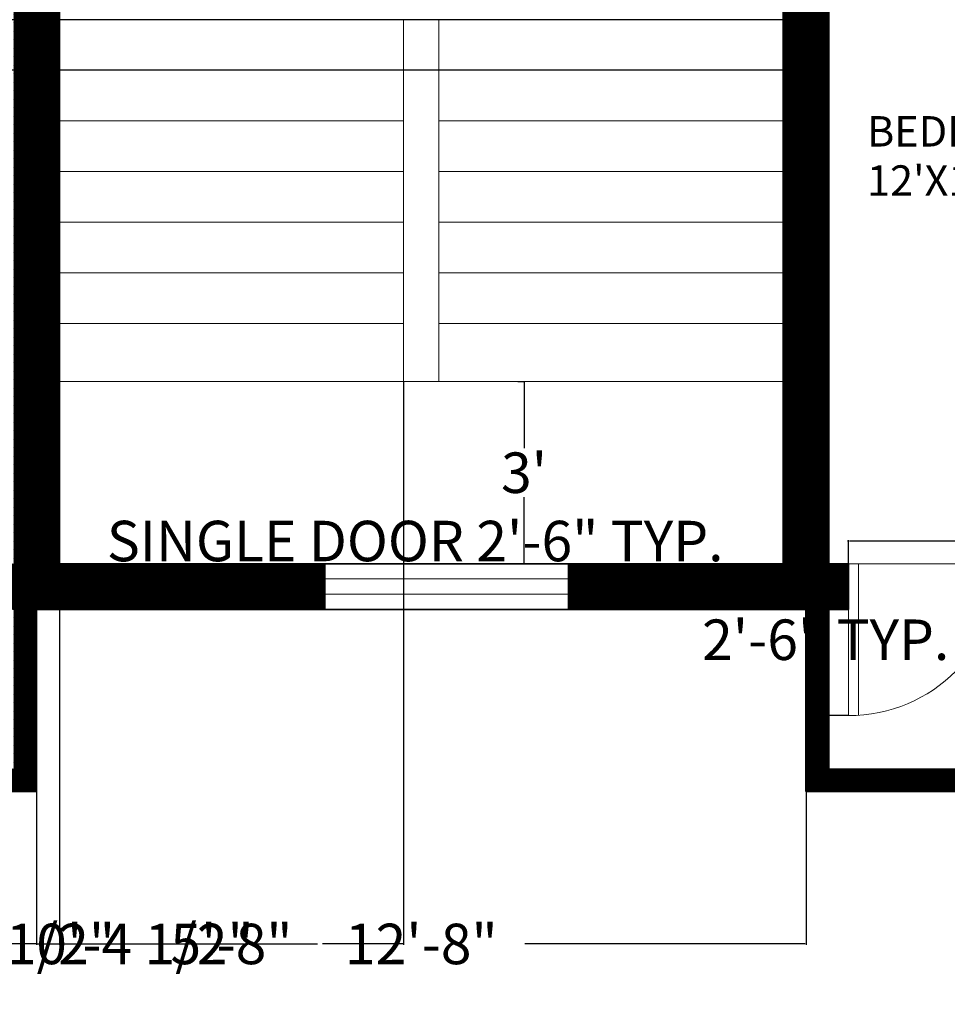
# Model space of a CAD drawing. Units: inches. Extents: x 108 to 771, y 58 to 590.
# Tile 3 of 8: x 341 to 524, y 58 to 253. Entities that reach past the tile are written whole.
import ezdxf

# ---------------------------------------------------------------- set-up
doc = ezdxf.new("R2010")
doc.units = ezdxf.units.IN
doc.header["$MEASUREMENT"] = 0
for name, color, linetype, lineweight in [('A-ANNO-DIMS', 2, 'Continuous', 13), ('A-AREA-IDEN', 7, 'Continuous', 18), ('A-DOOR', 3, 'Continuous', 18), ('A-FLOR-STRS', 7, 'Continuous', 18), ('A-GLAZ', 4, 'Continuous', 18), ('A-WALL', 7, 'Continuous', 35), ('A-WALL-PATT', 252, 'Continuous', 9)]:
    doc.layers.add(name, color=color, linetype=linetype, lineweight=lineweight)
doc.styles.get("Standard").update_dxf_attribs({"font": 'italic8.shx'})
doc.dimstyles.get("Standard").update_dxf_attribs({"dimtxt": 8, "dimasz": 0.18, "dimexe": 0.18, "dimexo": 0.0625, "dimgap": 0.09, "dimtad": 0, "dimtih": 1, "dimtoh": 1, "dimzin": 0, "dimdsep": 46, "dimlunit": 3, "dimtxsty": 'Standard', "dimcen": 0.09, "dimclrt": 6, "dimadec": 0, "dimazin": 0, "dimtfac": 1, "dimtofl": 0, "dimtmove": 0, "dimatfit": 3, "dimfxl": 1, "dimtolj": 1, "dimtzin": 0, "dimarcsym": 0})

# ---------------------------------------------------------------- blocks, each defined once
blk = doc.blocks.new('*D4')
at = {"layer": 'A-ANNO-DIMS', "color": 0, "lineweight": -2, "transparency": 16777216}
for p, q in [((438.9, 181.05), (440.33, 181.05)), ((440.15, 180.87), (440.15, 167.9)), ((440.15, 145.23), (440.15, 158.2)), ((438.9, 145.05), (440.33, 145.05))]:
    blk.add_line(p, q, dxfattribs=at)
at = {"layer": 'A-ANNO-DIMS', "color": 0, "transparency": 16777216}
for points in [[(440.12, 180.87), (440.18, 180.87), (440.15, 181.05)], [(440.12, 145.23), (440.18, 145.23), (440.15, 145.05)]]:
    blk.add_solid(points, dxfattribs=at)
at = {"layer": 'Defpoints', "color": 0, "transparency": 16777216}
for p in [(438.84, 181.05), (438.84, 145.05), (440.15, 145.05)]:
    blk.add_point(p, dxfattribs=at)
at = {"layer": 'A-ANNO-DIMS', "color": 0, "transparency": 16777216, "insert": (440.15, 163.05), "char_height": 8, "attachment_point": 5}
blk.add_mtext("\\A1;3'", dxfattribs=at)
blk = doc.blocks.new('DOOR-SINGLE-30')
for p, q in [((28, 29.93), (28, 0)), ((30, 30), (30, 0)), ((30, 0), (0, 0))]:
    blk.add_line(p, q)
blk.add_arc((30, 0), 30, 90, 180)
blk = doc.blocks.new('WINDOW-48')
for p, q in [((0, 48), (0, 0)), ((9, 48), (0, 48)), ((3, 48), (3, 0)), ((6, 48), (6, 0)), ((9, 0), (9, 48)), ((0, 0), (9, 0))]:
    blk.add_line(p, q)
blk = doc.blocks.new('*D24')
at = {"layer": 'A-ANNO-DIMS', "color": 0, "lineweight": -2, "transparency": 16777216}
for p, q in [((504.24, 149.55), (504.06, 149.55)), ((504.24, 145.12), (504.24, 149.73)), ((534.06, 149.55), (504.42, 149.55)), ((534.24, 145.12), (534.24, 149.73))]:
    blk.add_line(p, q, dxfattribs=at)
at = {"layer": 'A-ANNO-DIMS', "color": 0, "transparency": 16777216}
for points in [[(504.42, 149.58), (504.42, 149.52), (504.24, 149.55)], [(534.06, 149.58), (534.06, 149.52), (534.24, 149.55)]]:
    blk.add_solid(points, dxfattribs=at)
at = {"layer": 'Defpoints', "color": 0, "transparency": 16777216}
for p in [(504.24, 149.55), (504.24, 145.05), (534.24, 145.05)]:
    blk.add_point(p, dxfattribs=at)
at = {"layer": 'A-ANNO-DIMS', "color": 6, "transparency": 16777216, "insert": (418.64, 149.55), "char_height": 8, "attachment_point": 5}
blk.add_mtext('\\A1;SINGLE DOOR 2\'-6" TYP.', dxfattribs=at)
blk = doc.blocks.new('*D25')
at = {"layer": 'A-ANNO-DIMS', "color": 0, "lineweight": -2, "transparency": 16777216}
for p, q in [((504.18, 145.05), (499.56, 145.05)), ((499.74, 144.87), (499.74, 134.9)), ((499.74, 115.23), (499.74, 125.2)), ((504.18, 115.05), (499.56, 115.05))]:
    blk.add_line(p, q, dxfattribs=at)
at = {"layer": 'A-ANNO-DIMS', "color": 0, "transparency": 16777216}
for points in [[(499.71, 144.87), (499.77, 144.87), (499.74, 145.05)], [(499.71, 115.23), (499.77, 115.23), (499.74, 115.05)]]:
    blk.add_solid(points, dxfattribs=at)
at = {"layer": 'Defpoints', "color": 0, "transparency": 16777216}
for p in [(504.24, 145.05), (499.74, 115.05), (504.24, 115.05)]:
    blk.add_point(p, dxfattribs=at)
at = {"layer": 'A-ANNO-DIMS', "color": 6, "transparency": 16777216, "insert": (499.74, 130.05), "char_height": 8, "attachment_point": 5}
blk.add_mtext('\\A1;2\'-6" TYP.', dxfattribs=at)
blk = doc.blocks.new('*D46')
at = {"layer": 'A-ANNO-DIMS', "color": 0, "lineweight": -2, "transparency": 16777216}
for p, q in [((162.35, 99.99), (162.35, 69.77)), ((343.85, 99.99), (343.85, 69.77)), ((162.53, 69.95), (218.72, 69.95)), ((343.67, 69.95), (287.47, 69.95))]:
    blk.add_line(p, q, dxfattribs=at)
at = {"layer": 'A-ANNO-DIMS', "color": 0, "transparency": 16777216}
for points in [[(162.53, 69.98), (162.53, 69.92), (162.35, 69.95)], [(343.67, 69.98), (343.67, 69.92), (343.85, 69.95)]]:
    blk.add_solid(points, dxfattribs=at)
at = {"layer": 'Defpoints', "color": 0, "transparency": 16777216}
for p in [(162.35, 100.05), (343.85, 100.05), (343.85, 69.95)]:
    blk.add_point(p, dxfattribs=at)
at = {"layer": 'A-ANNO-DIMS', "color": 6, "transparency": 16777216, "insert": (253.1, 69.95), "char_height": 8, "attachment_point": 5}
blk.add_mtext('\\A1;15\'-1 1/2"', dxfattribs=at)
blk = doc.blocks.new('*D47')
at = {"layer": 'A-ANNO-DIMS', "color": 0, "lineweight": -2, "transparency": 16777216}
for p, q in [((343.85, 99.99), (343.85, 69.77)), ((495.85, 99.99), (495.85, 69.77)), ((344.03, 69.95), (399.37, 69.95)), ((495.67, 69.95), (440.32, 69.95))]:
    blk.add_line(p, q, dxfattribs=at)
at = {"layer": 'A-ANNO-DIMS', "color": 0, "transparency": 16777216}
for points in [[(344.03, 69.98), (344.03, 69.92), (343.85, 69.95)], [(495.67, 69.98), (495.67, 69.92), (495.85, 69.95)]]:
    blk.add_solid(points, dxfattribs=at)
at = {"layer": 'Defpoints', "color": 0, "transparency": 16777216}
for p in [(343.85, 100.05), (495.85, 100.05), (495.85, 69.95)]:
    blk.add_point(p, dxfattribs=at)
at = {"layer": 'A-ANNO-DIMS', "color": 6, "transparency": 16777216, "insert": (419.85, 69.95), "char_height": 8, "attachment_point": 5}
blk.add_mtext('\\A1;12\'-8"', dxfattribs=at)
blk = doc.blocks.new('*D52')
at = {"layer": 'A-ANNO-DIMS', "color": 0, "lineweight": -2, "transparency": 16777216}
for p, q in [((348.35, 145.12), (348.35, 578.33)), ((348.53, 578.15), (399.37, 578.15)), ((491.17, 578.15), (440.32, 578.15)), ((491.35, 145.12), (491.35, 578.33))]:
    blk.add_line(p, q, dxfattribs=at)
at = {"layer": 'A-ANNO-DIMS', "color": 0, "transparency": 16777216}
for points in [[(348.53, 578.18), (348.53, 578.12), (348.35, 578.15)], [(491.17, 578.18), (491.17, 578.12), (491.35, 578.15)]]:
    blk.add_solid(points, dxfattribs=at)
at = {"layer": 'Defpoints', "color": 0, "transparency": 16777216}
for p in [(491.35, 578.15), (348.35, 145.05), (491.35, 145.05)]:
    blk.add_point(p, dxfattribs=at)
at = {"layer": 'A-ANNO-DIMS', "color": 6, "transparency": 16777216, "insert": (419.85, 578.15), "char_height": 8, "attachment_point": 5}
blk.add_mtext('\\A1;11\'-11"', dxfattribs=at)
blk = doc.blocks.new('*D59')
at = {"layer": 'A-ANNO-DIMS', "color": 0, "lineweight": -2, "transparency": 16777216}
for p, q in [((327.35, 538.99), (327.35, 69.77)), ((331.85, 538.99), (331.85, 69.77)), ((327.53, 69.95), (331.67, 69.95)), ((331.85, 69.95), (332.03, 69.95))]:
    blk.add_line(p, q, dxfattribs=at)
at = {"layer": 'A-ANNO-DIMS', "color": 0, "transparency": 16777216}
for points in [[(327.53, 69.98), (327.53, 69.92), (327.35, 69.95)], [(331.67, 69.98), (331.67, 69.92), (331.85, 69.95)]]:
    blk.add_solid(points, dxfattribs=at)
at = {"layer": 'Defpoints', "color": 0, "transparency": 16777216}
for p in [(327.35, 539.05), (331.85, 539.05), (331.85, 69.95)]:
    blk.add_point(p, dxfattribs=at)
at = {"layer": 'A-ANNO-DIMS', "color": 6, "transparency": 16777216, "insert": (365.26, 69.95), "char_height": 8, "attachment_point": 5}
blk.add_mtext('\\A1;0\'-4 1/2"', dxfattribs=at)
blk = doc.blocks.new('*D61')
at = {"layer": 'A-ANNO-DIMS', "color": 0, "lineweight": -2, "transparency": 16777216}
for p, q in [((132.245389, 252.733083), (132.245389, 252.913083)), ((491.282889, 252.553083), (132.065389, 252.553083)), ((491.282889, 242.553083), (132.065389, 242.553083)), ((132.245389, 242.373083), (132.245389, 242.193083))]:
    blk.add_line(p, q, dxfattribs=at)
at = {"layer": 'A-ANNO-DIMS', "color": 0, "transparency": 16777216}
for points in [[(132.215389, 252.733083), (132.275389, 252.733083), (132.245389, 252.553083)], [(132.215389, 242.373083), (132.275389, 242.373083), (132.245389, 242.553083)]]:
    blk.add_solid(points, dxfattribs=at)
at = {"layer": 'Defpoints', "color": 0, "transparency": 16777216}
for p in [(491.345389, 252.553083), (132.245389, 242.553083), (491.345389, 242.553083)]:
    blk.add_point(p, dxfattribs=at)
at = {"layer": 'A-ANNO-DIMS', "color": 6, "transparency": 16777216, "insert": (132.245389, 247.553083), "char_height": 8, "attachment_point": 5}
blk.add_mtext('\\A1;0\'-10"', dxfattribs=at)
blk = doc.blocks.new('*D66')
at = {"layer": 'A-ANNO-DIMS', "color": 0, "lineweight": -2, "transparency": 16777216}
for p, q in [((348.35, 180.99), (348.35, 69.77)), ((416.35, 180.99), (416.35, 69.77)), ((348.53, 69.95), (364.35, 69.95)), ((416.17, 69.95), (400.34, 69.95))]:
    blk.add_line(p, q, dxfattribs=at)
at = {"layer": 'A-ANNO-DIMS', "color": 0, "transparency": 16777216}
for points in [[(348.53, 69.98), (348.53, 69.92), (348.35, 69.95)], [(416.17, 69.98), (416.17, 69.92), (416.35, 69.95)]]:
    blk.add_solid(points, dxfattribs=at)
at = {"layer": 'Defpoints', "color": 0, "transparency": 16777216}
for p in [(348.35, 181.05), (416.35, 181.05), (416.35, 69.95)]:
    blk.add_point(p, dxfattribs=at)
at = {"layer": 'A-ANNO-DIMS', "color": 6, "transparency": 16777216, "insert": (382.35, 69.95), "char_height": 8, "attachment_point": 5}
blk.add_mtext('\\A1;5\'-8"', dxfattribs=at)
blk = doc.blocks.new('*D68')
at = {"layer": 'A-ANNO-DIMS', "color": 0, "lineweight": -2, "transparency": 16777216}
for p, q in [((259.84, 135.99), (259.84, 69.77)), ((304.47, 135.99), (304.47, 69.77)), ((260.02, 69.95), (304.29, 69.95)), ((304.47, 69.95), (304.65, 69.95))]:
    blk.add_line(p, q, dxfattribs=at)
at = {"layer": 'A-ANNO-DIMS', "color": 0, "transparency": 16777216}
for points in [[(260.02, 69.98), (260.02, 69.92), (259.84, 69.95)], [(304.29, 69.98), (304.29, 69.92), (304.47, 69.95)]]:
    blk.add_solid(points, dxfattribs=at)
at = {"layer": 'Defpoints', "color": 0, "transparency": 16777216}
for p in [(259.84, 136.05), (304.47, 136.05), (304.47, 69.95)]:
    blk.add_point(p, dxfattribs=at)
at = {"layer": 'A-ANNO-DIMS', "color": 6, "transparency": 16777216, "insert": (337.88, 69.95), "char_height": 8, "attachment_point": 5}
blk.add_mtext('\\A1;3\'-8 1/2"', dxfattribs=at)

msp = doc.modelspace()

# ---------------------------------------------------------------- hatches: boundary and pattern name
at = {"layer": 'A-WALL-PATT'}
h = msp.add_hatch(dxfattribs=at)
h.set_pattern_fill('ANSI31', color=256)
h.paths.add_polyline_path([(171.345, 461.548), (162.345, 461.548), (162.345, 390.901), (171.345, 390.901), (171.345, 393.51), (171.345, 402.553), (233.142, 402.553), (233.142, 407.053), (171.345, 407.053)])
h.paths.add_polyline_path([(331.845, 438.553), (336.68, 438.554), (336.68, 443.053), (331.845, 443.053), (331.845, 539.053), (365.02, 539.053), (365.02, 548.053), (280.772, 548.053), (280.772, 539.053), (327.345, 539.053), (327.345, 407.053), (325.63, 407.053), (325.63, 402.553), (331.845, 402.553)])
h.paths.add_polyline_path([(286.63, 407.053), (263.142, 407.053), (263.142, 402.553), (267.345, 402.553), (267.345, 352.303), (171.345, 352.303), (171.345, 360.901), (162.345, 360.901), (162.345, 336.026), (171.345, 336.026), (171.345, 347.803), (267.345, 347.803), (267.345, 293.053), (263.142, 293.053), (263.142, 288.553), (293.037, 288.553), (293.037, 293.053), (271.845, 293.053), (271.845, 402.553), (286.63, 402.553)])
h.paths.add_polyline_path([(466.018, 443.053), (424.345, 443.053), (424.345, 539.053), (453.584, 539.053), (453.584, 548.053), (395.02, 548.053), (395.02, 539.053), (419.845, 539.053), (420.71, 443.053), (372.68, 443.053), (372.68, 438.557), (420.751, 438.561), (421.075, 402.553), (422.061, 293.053), (419.994, 293.053), (419.994, 288.553), (426.124, 288.553), (426.124, 293.053), (424.345, 293.053), (424.345, 402.553), (424.345, 438.553), (466.018, 438.553)])
h.paths.add_polyline_path([(512.345, 539.053), (583.918, 539.053), (583.918, 548.053), (483.584, 548.053), (483.584, 539.053), (507.845, 539.053), (507.845, 443.053), (502.018, 443.053), (502.018, 438.553), (507.845, 438.553), (507.845, 402.553), (515.658, 402.553), (515.658, 407.053), (512.345, 407.053)])
h.paths.add_polyline_path([(232.772, 548.053), (162.345, 548.053), (162.345, 509.548), (171.345, 509.548), (171.345, 539.053), (232.772, 539.053)])
h.paths.add_polyline_path([(233.142, 293.053), (171.345, 293.053), (171.345, 306.026), (162.345, 306.026), (162.345, 230.8), (171.345, 230.8), (171.345, 288.553), (233.142, 288.553)])
h.paths.add_polyline_path([(359.994, 293.053), (332.037, 293.053), (332.037, 288.553), (339.345, 288.553), (339.345, 145.053), (334.469, 145.053), (334.469, 136.053), (339.345, 136.053), (339.345, 104.553), (166.845, 104.553), (166.845, 136.053), (211.837, 136.053), (211.837, 145.053), (171.345, 145.053), (171.345, 182.8), (162.345, 182.8), (162.345, 100.053), (343.845, 100.053), (343.845, 136.053), (400.886, 136.053), (400.886, 145.053), (348.345, 145.053), (348.345, 288.553), (359.994, 288.553)])
h.paths.add_polyline_path([(500.345, 288.553), (503.755, 288.553), (503.755, 293.053), (486.124, 293.053), (486.124, 288.553), (491.345, 288.553), (491.345, 145.053), (448.886, 145.053), (448.886, 136.053), (495.845, 136.053), (495.845, 100.053), (677.345, 100.053), (677.345, 186.265), (668.345, 186.265), (668.345, 145.053), (627.637, 145.053), (627.637, 136.053), (672.845, 136.053), (672.845, 104.278), (500.345, 104.539), (500.345, 136.053), (504.239, 136.053), (504.239, 145.053), (500.345, 145.053)])
h.paths.add_polyline_path([(580.913, 293.053), (572.345, 293.053), (572.345, 347.803), (668.345, 347.803), (668.345, 330.831), (677.345, 330.831), (677.345, 366.853), (668.345, 366.853), (668.345, 352.303), (572.345, 352.303), (572.345, 402.553), (580.418, 402.553), (580.418, 407.053), (554.658, 407.053), (554.658, 402.553), (567.845, 402.553), (567.845, 293.053), (542.755, 293.053), (542.755, 288.553), (580.913, 288.553)])
h.paths.add_polyline_path([(677.345, 300.831), (668.345, 300.831), (668.345, 293.053), (610.913, 293.053), (610.913, 288.553), (668.345, 288.553), (668.345, 234.265), (677.345, 234.265)])
h.paths.add_polyline_path([(304.469, 145.053), (259.837, 145.053), (259.837, 136.053), (304.469, 136.053)], flags=17)
h.paths.add_polyline_path([(579.637, 145.053), (534.239, 145.053), (534.239, 136.053), (579.637, 136.053)], flags=17)
h.paths.add_polyline_path([(677.345, 450.416), (668.345, 450.416), (668.345, 407.053), (610.418, 407.053), (610.418, 402.553), (668.345, 402.553), (668.345, 396.853), (677.345, 396.853)])
h.paths.add_polyline_path([(677.345, 548.053), (631.918, 548.053), (631.918, 539.053), (668.345, 539.053), (668.345, 498.416), (677.345, 498.416)])
h = msp.add_hatch(dxfattribs=at)
h.set_pattern_fill('ANSI31', color=256)
h.paths.add_polyline_path([(365.02, 548.053), (280.772, 548.053), (280.772, 539.053), (327.345, 539.053), (327.345, 407.053), (325.63, 407.053), (325.63, 402.553), (331.845, 402.553), (331.845, 438.553), (336.68, 438.554), (336.68, 443.053), (331.845, 443.053), (331.845, 539.053), (365.02, 539.053)])
h.paths.add_polyline_path([(453.584, 548.053), (395.02, 548.053), (395.02, 539.053), (419.845, 539.053), (420.71, 443.053), (372.68, 443.053), (372.68, 438.557), (420.751, 438.561), (421.075, 402.553), (422.061, 293.053), (419.994, 293.053), (419.994, 288.553), (426.124, 288.553), (426.124, 293.053), (424.345, 293.053), (424.345, 402.553), (424.345, 438.553), (466.018, 438.553), (466.018, 443.053), (424.345, 443.053), (424.345, 539.053), (453.584, 539.053)])
h.paths.add_polyline_path([(232.772, 548.053), (162.345, 548.053), (162.345, 509.548), (171.345, 509.548), (171.345, 539.053), (232.772, 539.053)])
h.paths.add_polyline_path([(171.345, 461.548), (162.345, 461.548), (162.345, 390.901), (171.345, 390.901), (171.345, 393.51), (171.345, 402.553), (233.142, 402.553), (233.142, 407.053), (171.345, 407.053)])
h.paths.add_polyline_path([(286.63, 407.053), (263.142, 407.053), (263.142, 402.553), (267.345, 402.553), (267.345, 352.303), (171.345, 352.303), (171.345, 360.901), (162.345, 360.901), (162.345, 336.026), (171.345, 336.026), (171.345, 347.803), (267.345, 347.803), (267.345, 293.053), (263.142, 293.053), (263.142, 288.553), (293.037, 288.553), (293.037, 293.053), (271.845, 293.053), (271.845, 402.553), (286.63, 402.553)])
h.paths.add_polyline_path([(171.345, 306.026), (162.345, 306.026), (162.345, 230.8), (171.345, 230.8), (171.345, 288.553), (233.142, 288.553), (233.142, 293.053), (171.345, 293.053)])
h.paths.add_polyline_path([(348.345, 288.553), (359.994, 288.553), (359.994, 293.053), (332.037, 293.053), (332.037, 288.553), (339.345, 288.553), (339.345, 145.053), (334.469, 145.053), (334.469, 136.053), (339.345, 136.053), (339.345, 104.553), (166.845, 104.553), (166.845, 136.053), (211.837, 136.053), (211.837, 145.053), (171.345, 145.053), (171.345, 182.8), (162.345, 182.8), (162.345, 100.053), (343.845, 100.053), (343.845, 136.053), (400.886, 136.053), (400.886, 145.053), (348.345, 145.053)])
h.paths.add_polyline_path([(503.755, 293.053), (486.124, 293.053), (486.124, 288.553), (491.345, 288.553), (491.345, 145.053), (448.886, 145.053), (448.886, 136.053), (495.845, 136.053), (495.845, 100.053), (677.345, 100.053), (677.345, 186.265), (668.345, 186.265), (668.345, 145.053), (627.637, 145.053), (627.637, 136.053), (672.845, 136.053), (672.845, 104.278), (500.345, 104.539), (500.345, 136.053), (504.239, 136.053), (504.239, 145.053), (500.345, 145.053), (500.345, 288.553), (503.755, 288.553)])
h.paths.add_polyline_path([(580.913, 293.053), (572.345, 293.053), (572.345, 347.803), (668.345, 347.803), (668.345, 330.831), (677.345, 330.831), (677.345, 366.853), (668.345, 366.853), (668.345, 352.303), (572.345, 352.303), (572.345, 402.553), (580.418, 402.553), (580.418, 407.053), (554.658, 407.053), (554.658, 402.553), (567.845, 402.553), (567.845, 293.053), (542.755, 293.053), (542.755, 288.553), (580.913, 288.553)])
h.paths.add_polyline_path([(677.345, 300.831), (668.345, 300.831), (668.345, 293.053), (610.913, 293.053), (610.913, 288.553), (668.345, 288.553), (668.345, 234.265), (677.345, 234.265)])
h.paths.add_polyline_path([(579.637, 145.053), (534.239, 145.053), (534.239, 136.053), (579.637, 136.053)], flags=17)
h.paths.add_polyline_path([(304.469, 145.053), (259.837, 145.053), (259.837, 136.053), (304.469, 136.053)], flags=17)
h.paths.add_polyline_path([(583.918, 548.053), (483.584, 548.053), (483.584, 539.053), (507.845, 539.053), (507.845, 443.053), (502.018, 443.053), (502.018, 438.553), (507.845, 438.553), (507.845, 402.553), (515.658, 402.553), (515.658, 407.053), (512.345, 407.053), (512.345, 539.053), (583.918, 539.053)])
h.paths.add_polyline_path([(677.345, 548.053), (631.918, 548.053), (631.918, 539.053), (668.345, 539.053), (668.345, 498.416), (677.345, 498.416)])
h.paths.add_polyline_path([(677.345, 450.416), (668.345, 450.416), (668.345, 407.053), (610.418, 407.053), (610.418, 402.553), (668.345, 402.553), (668.345, 396.853), (677.345, 396.853)])

# ---------------------------------------------------------------- linework, layer by layer
at = {"layer": 'A-FLOR-STRS'}
for p, q in [((491.345, 252.553), (348.345, 252.553)), ((416.345, 181.053), (416.345, 252.553)), ((423.345, 252.553), (423.345, 181.053)), ((416.345, 242.553), (348.345, 242.553)), ((491.345, 242.553), (423.345, 242.553)), ((416.345, 232.553), (348.345, 232.553)), ((491.345, 232.553), (423.345, 232.553)), ((416.345, 222.553), (348.345, 222.553)), ((491.345, 222.553), (423.345, 222.553)), ((416.345, 212.553), (348.345, 212.553)), ((491.345, 212.553), (423.345, 212.553)), ((416.345, 202.553), (348.345, 202.553)), ((491.345, 202.553), (423.345, 202.553)), ((416.345, 192.553), (348.345, 192.553)), ((491.345, 192.553), (423.345, 192.553)), ((491.345, 181.053), (348.345, 181.053))]:
    msp.add_line(p, q, dxfattribs=at)
at = {"layer": 'A-WALL'}
for p, q in [((348.345, 145.053), (348.345, 288.553)), ((491.345, 288.553), (491.345, 145.053)), ((500.345, 288.553), (500.345, 145.053)), ((491.345, 145.053), (348.345, 145.053)), ((504.239, 145.053), (500.345, 145.053)), ((504.239, 136.053), (504.239, 145.053)), ((495.845, 136.053), (343.845, 136.053)), ((343.845, 100.053), (343.845, 136.053)), ((495.845, 136.053), (495.845, 100.053)), ((500.345, 136.053), (500.345, 104.539)), ((504.239, 136.053), (500.345, 136.053)), ((672.845, 104.278), (500.345, 104.539)), ((343.845, 100.053), (162.345, 100.053)), ((677.345, 100.053), (495.845, 100.053))]:
    msp.add_line(p, q, dxfattribs=at)

# ---------------------------------------------------------------- block references
at = {"layer": 'A-DOOR', "rotation": 180}
msp.add_blockref('DOOR-SINGLE-30', (534.239, 145.053), dxfattribs=at)
at = {"layer": 'A-GLAZ', "rotation": 269.9999999999995}
msp.add_blockref('WINDOW-48', (400.887, 145.053), dxfattribs=at)

# ---------------------------------------------------------------- texts
at = {"layer": 'A-AREA-IDEN'}
for s, p in [('BEDROOM', (507.917, 227.496)), ("12'X12'", (507.917, 217.781))]:
    msp.add_text(s, height=6, dxfattribs=at).set_placement(p)

# ---------------------------------------------------------------- dimensions: what is measured, and where the dimension line sits
at = {"layer": 'A-ANNO-DIMS'}
for base, p1, p2, picture, middle in [((491.345, 578.153), (348.345, 145.053), (491.345, 145.053), '*D52', (419.845, 578.153)), ((331.845, 69.953), (327.345, 539.053), (331.845, 539.053), '*D59', (365.258, 69.953)), ((416.345, 69.953), (348.345, 181.053), (416.345, 181.053), '*D66', (382.345, 69.953)), ((304.469, 69.953), (259.837, 136.053), (304.469, 136.053), '*D68', (337.882, 69.953)), ((343.845, 69.953), (162.345, 100.053), (343.845, 100.053), '*D46', (253.095, 69.953)), ((495.845, 69.953), (343.845, 100.053), (495.845, 100.053), '*D47', (419.845, 69.953))]:
    dim = msp.add_linear_dim(base=base, p1=p1, p2=p2, dimstyle='Standard', override={"dimdec": 1, "dimlfac": 1, "dimrnd": 0, "dimzin": 1, "dimdsep": 46, "dimlunit": 4, "dimfrac": 2}, dxfattribs=at)
    dim.commit()
    dim.dimension.update_dxf_attribs({"geometry": picture, "text_midpoint": middle})
for base, p1, p2, override, picture, middle in [((132.245, 242.553), (491.345, 252.553), (491.345, 242.553), {"dimdec": 1, "dimlfac": 1, "dimrnd": 0, "dimzin": 1, "dimdsep": 46, "dimlunit": 4, "dimfrac": 2}, '*D61', (132.245, 247.553)), ((440.153, 145.053), (438.84, 181.053), (438.84, 145.053), {"dimclrd": 0, "dimclre": 0, "dimclrt": 0}, '*D4', (440.153, 163.053))]:
    dim = msp.add_linear_dim(base=base, p1=p1, p2=p2, angle=90, dimstyle='Standard', override=override, dxfattribs=at)
    dim.commit()
    dim.dimension.update_dxf_attribs({"geometry": picture, "text_midpoint": middle})
for base, p1, p2, angle, text, picture, middle in [((504.239, 149.553), (534.239, 145.053), (504.239, 145.053), 180, 'SINGLE DOOR <> TYP.', '*D24', (418.635, 149.553)), ((499.739, 115.053), (504.239, 145.053), (504.239, 115.053), 270, '<> TYP.', '*D25', (499.739, 130.053))]:
    dim = msp.add_linear_dim(base=base, p1=p1, p2=p2, angle=angle, text=text, dimstyle='Standard', override={"dimdec": 1, "dimlfac": 1, "dimrnd": 0, "dimzin": 1, "dimdsep": 46, "dimlunit": 4, "dimfrac": 2}, dxfattribs=at)
    dim.commit()
    dim.dimension.update_dxf_attribs({"geometry": picture, "text_midpoint": middle})

doc.saveas('drawing.dxf')
